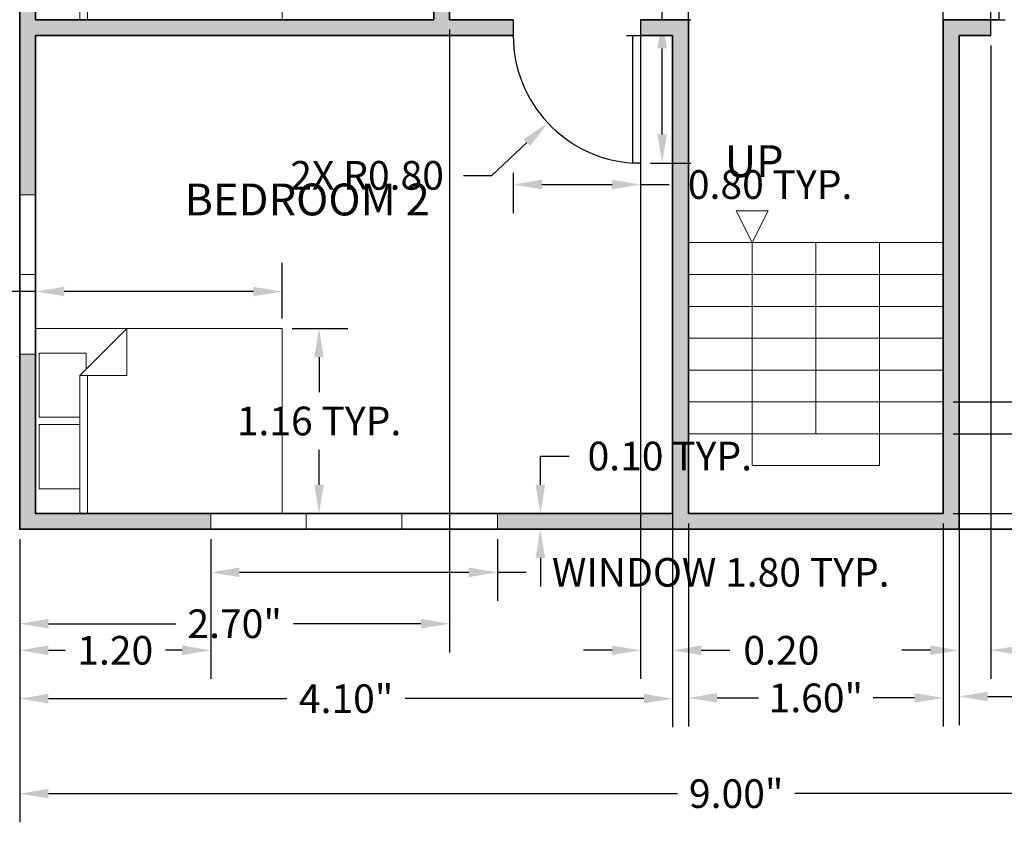
# Model space of a CAD drawing. Units: metres. Extents: x -1.9 to 13.1, y 0.9 to 14.8.
# Tile 2 of 7: x 1.2 to 7.4, y 0.9 to 5.9. Entities that reach past the tile are written whole.
import ezdxf

# ---------------------------------------------------------------- set-up
doc = ezdxf.new("R2010")
doc.units = ezdxf.units.M
doc.header["$MEASUREMENT"] = 0
for name, color, linetype, lineweight in [('A-ANNO-DIMS', 2, 'Continuous', 13), ('A-ANNO-SYMB', 7, 'Continuous', 18), ('A-ANNO-TEXT', 7, 'Continuous', 18), ('A-AREA-IDEN', 7, 'Continuous', 25), ('A-DOOR', 3, 'Continuous', 25), ('A-FLOR-STRS', 7, 'Continuous', 18), ('A-FURN', 8, 'Continuous', 18), ('A-GLAZ', 4, 'Continuous', 18), ('A-WALL', 7, 'Continuous', 35), ('A-WALL-PATT', 252, 'Continuous', 13)]:
    doc.layers.add(name, color=color, linetype=linetype, lineweight=lineweight)
doc.styles.get("Standard").update_dxf_attribs({"font": 'arial.ttf'})
doc.dimstyles.get("Standard").update_dxf_attribs({"dimtxt": 0.18, "dimasz": 0.18, "dimexe": 0.18, "dimexo": 0.0625, "dimgap": 0.09, "dimtad": 0, "dimtih": 1, "dimtoh": 1, "dimzin": 0, "dimdsep": 46, "dimlunit": 3, "dimtxsty": 'Standard', "dimcen": 0.09, "dimadec": 0, "dimazin": 0, "dimtfac": 1, "dimtofl": 0, "dimtmove": 0, "dimatfit": 3, "dimfxl": 1, "dimtolj": 1, "dimtzin": 0, "dimarcsym": 0})

# ---------------------------------------------------------------- blocks, each defined once
blk = doc.blocks.new('Bed - Queen')
for p, q in [((0, -80.00003), (0, 0)), ((0, 0), (59.99999, 0)), ((59.99999, 0), (59.99999, -80.00003)), ((7.99999, -1.2), (28.79998, -1.2)), ((7.99999, -14.4), (7.99999, -1.2)), ((28.79998, -1.2), (28.79998, -14.4)), ((31.19999, -1.2), (51.99999, -1.2)), ((31.19999, -14.4), (31.19999, -1.2)), ((51.99999, -1.2), (51.99999, -16.4)), ((0, -14.4), (44.8, -14.4)), ((59.99999, -29.6), (44.8, -14.4)), ((44.8, -14.4), (44.8, -29.6)), ((44.8, -16.8), (0, -16.8)), ((51.99999, -16.4), (46.79936, -16.4)), ((44.8, -29.6), (59.99999, -29.6)), ((59.99999, -80.00003), (0, -80.00003))]:
    blk.add_line(p, q)
blk = doc.blocks.new('*D8')
at = {"layer": 'A-ANNO-DIMS', "color": 0, "lineweight": -2, "transparency": 16777216}
for p, q in [((3.9038, 5.8339), (3.9038, 1.9238)), ((1.2038, 2.6339), (1.2038, 1.9238)), ((1.3838, 2.1038), (2.1841, 2.1038)), ((3.7238, 2.1038), (2.9236, 2.1038))]:
    blk.add_line(p, q, dxfattribs=at)
at = {"layer": 'A-ANNO-DIMS', "color": 0, "transparency": 16777216}
for points in [[(1.3838, 2.1338), (1.3838, 2.0738), (1.2038, 2.1038)], [(3.7238, 2.1338), (3.7238, 2.0738), (3.9038, 2.1038)]]:
    blk.add_solid(points, dxfattribs=at)
at = {"layer": 'Defpoints', "color": 0, "transparency": 16777216}
for p in [(3.9038, 5.8964), (1.2038, 2.6964), (3.9038, 2.1038)]:
    blk.add_point(p, dxfattribs=at)
at = {"layer": 'A-ANNO-DIMS', "color": 0, "transparency": 16777216, "insert": (2.5538, 2.1038), "char_height": 0.18, "attachment_point": 5}
blk.add_mtext('\\A1;2.70"', dxfattribs=at)
blk = doc.blocks.new('*D9')
at = {"layer": 'A-ANNO-DIMS', "color": 0, "lineweight": -2, "transparency": 16777216}
for p, q in [((5.3038, 2.7339), (5.3038, 1.4532)), ((1.2038, 2.6339), (1.2038, 1.4532)), ((1.3838, 1.6332), (2.882, 1.6332)), ((5.1238, 1.6332), (3.6257, 1.6332))]:
    blk.add_line(p, q, dxfattribs=at)
at = {"layer": 'A-ANNO-DIMS', "color": 0, "transparency": 16777216}
for points in [[(1.3838, 1.6632), (1.3838, 1.6032), (1.2038, 1.6332)], [(5.1238, 1.6632), (5.1238, 1.6032), (5.3038, 1.6332)]]:
    blk.add_solid(points, dxfattribs=at)
at = {"layer": 'Defpoints', "color": 0, "transparency": 16777216}
for p in [(5.3038, 2.7964), (1.2038, 2.6964), (5.3038, 1.6332)]:
    blk.add_point(p, dxfattribs=at)
at = {"layer": 'A-ANNO-DIMS', "color": 0, "transparency": 16777216, "insert": (3.2538, 1.6332), "char_height": 0.18, "attachment_point": 5}
blk.add_mtext('\\A1;4.10"', dxfattribs=at)
blk = doc.blocks.new('*D10')
at = {"layer": 'A-ANNO-DIMS', "color": 0, "lineweight": -2, "transparency": 16777216}
for p, q in [((5.4038, 2.7339), (5.4038, 1.4582)), ((7.0038, 2.7339), (7.0038, 1.4582)), ((5.5838, 1.6382), (5.8441, 1.6382)), ((6.8238, 1.6382), (6.5636, 1.6382))]:
    blk.add_line(p, q, dxfattribs=at)
at = {"layer": 'A-ANNO-DIMS', "color": 0, "transparency": 16777216}
for points in [[(5.5838, 1.6682), (5.5838, 1.6082), (5.4038, 1.6382)], [(6.8238, 1.6682), (6.8238, 1.6082), (7.0038, 1.6382)]]:
    blk.add_solid(points, dxfattribs=at)
at = {"layer": 'Defpoints', "color": 0, "transparency": 16777216}
for p in [(5.4038, 2.7964), (7.0038, 2.7964), (7.0038, 1.6382)]:
    blk.add_point(p, dxfattribs=at)
at = {"layer": 'A-ANNO-DIMS', "color": 0, "transparency": 16777216, "insert": (6.2038, 1.6382), "char_height": 0.18, "attachment_point": 5}
blk.add_mtext('\\A1;1.60"', dxfattribs=at)
blk = doc.blocks.new('*D11')
at = {"layer": 'A-ANNO-DIMS', "color": 0, "lineweight": -2, "transparency": 16777216}
for p, q in [((7.1038, 2.6339), (7.1038, 1.467)), ((10.2038, 2.6339), (10.2038, 1.467)), ((7.2838, 1.647), (8.2857, 1.647)), ((10.0238, 1.647), (9.022, 1.647))]:
    blk.add_line(p, q, dxfattribs=at)
at = {"layer": 'A-ANNO-DIMS', "color": 0, "transparency": 16777216}
for points in [[(7.2838, 1.677), (7.2838, 1.617), (7.1038, 1.647)], [(10.0238, 1.677), (10.0238, 1.617), (10.2038, 1.647)]]:
    blk.add_solid(points, dxfattribs=at)
at = {"layer": 'Defpoints', "color": 0, "transparency": 16777216}
for p in [(7.1038, 2.6964), (10.2038, 2.6964), (10.2038, 1.647)]:
    blk.add_point(p, dxfattribs=at)
at = {"layer": 'A-ANNO-DIMS', "color": 0, "transparency": 16777216, "insert": (8.6538, 1.647), "char_height": 0.18, "attachment_point": 5}
blk.add_mtext('\\A1;3.10"', dxfattribs=at)
blk = doc.blocks.new('*D12')
at = {"layer": 'A-ANNO-DIMS', "color": 0, "lineweight": -2, "transparency": 16777216}
for p, q in [((1.2038, 2.6339), (1.2038, 0.8568)), ((10.2038, 2.6339), (10.2038, 0.8568)), ((1.3838, 1.0368), (5.3356, 1.0368)), ((10.0238, 1.0368), (6.0721, 1.0368))]:
    blk.add_line(p, q, dxfattribs=at)
at = {"layer": 'A-ANNO-DIMS', "color": 0, "transparency": 16777216}
for points in [[(1.3838, 1.0668), (1.3838, 1.0068), (1.2038, 1.0368)], [(10.0238, 1.0668), (10.0238, 1.0068), (10.2038, 1.0368)]]:
    blk.add_solid(points, dxfattribs=at)
at = {"layer": 'Defpoints', "color": 0, "transparency": 16777216}
for p in [(1.2038, 2.6964), (10.2038, 2.6964), (10.2038, 1.0368)]:
    blk.add_point(p, dxfattribs=at)
at = {"layer": 'A-ANNO-DIMS', "color": 0, "transparency": 16777216, "insert": (5.7038, 1.0368), "char_height": 0.18, "attachment_point": 5}
blk.add_mtext('\\A1;9.00"', dxfattribs=at)
blk = doc.blocks.new('*D13')
at = {"layer": 'A-ANNO-DIMS', "color": 0, "lineweight": -2, "transparency": 16777216}
for p, q in [((7.1663, 13.6964), (12.9272, 13.6964)), ((12.7472, 13.5164), (12.7472, 8.3783)), ((12.7472, 2.8764), (12.7472, 8.0145)), ((10.2663, 2.6964), (12.9272, 2.6964))]:
    blk.add_line(p, q, dxfattribs=at)
at = {"layer": 'A-ANNO-DIMS', "color": 0, "transparency": 16777216}
for points in [[(12.7172, 13.5164), (12.7772, 13.5164), (12.7472, 13.6964)], [(12.7172, 2.8764), (12.7772, 2.8764), (12.7472, 2.6964)]]:
    blk.add_solid(points, dxfattribs=at)
at = {"layer": 'Defpoints', "color": 0, "transparency": 16777216}
for p in [(7.1038, 13.6964), (12.7472, 13.6964), (10.2038, 2.6964)]:
    blk.add_point(p, dxfattribs=at)
at = {"layer": 'A-ANNO-DIMS', "color": 0, "transparency": 16777216, "insert": (12.7472, 8.1964), "char_height": 0.18, "attachment_point": 5}
blk.add_mtext('\\A1;11.00"', dxfattribs=at)
blk = doc.blocks.new('*D20')
at = {"layer": 'A-ANNO-DIMS', "color": 0, "lineweight": -2, "transparency": 16777216}
for p, q in [((1.1413, 10.5964), (-1.7723, 10.5964)), ((-1.5923, 10.4164), (-1.5923, 6.8283)), ((-1.5923, 2.8764), (-1.5923, 6.4645)), ((1.1413, 2.6964), (-1.7723, 2.6964))]:
    blk.add_line(p, q, dxfattribs=at)
at = {"layer": 'A-ANNO-DIMS', "color": 0, "transparency": 16777216}
for points in [[(-1.6223, 10.4164), (-1.5623, 10.4164), (-1.5923, 10.5964)], [(-1.6223, 2.8764), (-1.5623, 2.8764), (-1.5923, 2.6964)]]:
    blk.add_solid(points, dxfattribs=at)
at = {"layer": 'Defpoints', "color": 0, "transparency": 16777216}
for p in [(1.2038, 10.5964), (-1.5923, 2.6964), (1.2038, 2.6964)]:
    blk.add_point(p, dxfattribs=at)
at = {"layer": 'A-ANNO-DIMS', "color": 0, "transparency": 16777216, "insert": (-1.5923, 6.6464), "char_height": 0.18, "attachment_point": 5}
blk.add_mtext('\\A1;7.90"', dxfattribs=at)
blk = doc.blocks.new('*D22')
at = {"layer": 'A-ANNO-DIMS', "color": 0, "lineweight": -2, "transparency": 16777216}
for p, q in [((1.1413, 9.2964), (-0.3896, 9.2964)), ((-0.2096, 9.1164), (-0.2096, 7.7756)), ((-0.2096, 6.0709), (-0.2096, 7.4117)), ((1.1413, 5.8909), (-0.3896, 5.8909))]:
    blk.add_line(p, q, dxfattribs=at)
at = {"layer": 'A-ANNO-DIMS', "color": 0, "transparency": 16777216}
for points in [[(-0.2396, 9.1164), (-0.1796, 9.1164), (-0.2096, 9.2964)], [(-0.2396, 6.0709), (-0.1796, 6.0709), (-0.2096, 5.8909)]]:
    blk.add_solid(points, dxfattribs=at)
at = {"layer": 'Defpoints', "color": 0, "transparency": 16777216}
for p in [(1.2038, 9.2964), (-0.2096, 5.8909), (1.2038, 5.8909)]:
    blk.add_point(p, dxfattribs=at)
at = {"layer": 'A-ANNO-DIMS', "color": 0, "transparency": 16777216, "insert": (-0.2096, 7.5936), "char_height": 0.18, "attachment_point": 5}
blk.add_mtext('\\A1;3.41"', dxfattribs=at)
blk = doc.blocks.new('*D23')
at = {"layer": 'A-ANNO-DIMS', "color": 0, "lineweight": -2, "transparency": 16777216}
for p, q in [((1.1413, 5.7874), (-0.4098, 5.7874)), ((-0.2298, 5.6074), (-0.2298, 4.4239)), ((-0.2298, 2.8764), (-0.2298, 4.0599)), ((1.1413, 2.6964), (-0.4098, 2.6964))]:
    blk.add_line(p, q, dxfattribs=at)
at = {"layer": 'A-ANNO-DIMS', "color": 0, "transparency": 16777216}
for points in [[(-0.2598, 5.6074), (-0.1998, 5.6074), (-0.2298, 5.7874)], [(-0.2598, 2.8764), (-0.1998, 2.8764), (-0.2298, 2.6964)]]:
    blk.add_solid(points, dxfattribs=at)
at = {"layer": 'Defpoints', "color": 0, "transparency": 16777216}
for p in [(1.2038, 5.7874), (-0.2298, 2.6964), (1.2038, 2.6964)]:
    blk.add_point(p, dxfattribs=at)
at = {"layer": 'A-ANNO-DIMS', "color": 0, "transparency": 16777216, "insert": (-0.2298, 4.2419), "char_height": 0.18, "attachment_point": 5}
blk.add_mtext('\\A1;3.09"', dxfattribs=at)
blk = doc.blocks.new('DOOR-800')
for p, q in [((0, 0.9), (0, 0.8)), ((0.8, 0.9), (0.8, 0.8)), ((0.75, 0), (0.75, 0.8)), ((0.75, 0.8), (0.8, 0.8)), ((0.8, 0.8), (0.8, 0)), ((0.8, 0), (0.75, 0))]:
    blk.add_line(p, q)
blk.add_arc((0.8017, 0.8), 0.8017, 180, 266.30478)
blk = doc.blocks.new('WIN-1000')
for p, q in [((0.1, 1), (0, 1)), ((0.1, 0.5), (0, 0.5)), ((0.1, 0), (0, 0))]:
    blk.add_line(p, q)
blk = doc.blocks.new('WIN-1800')
for p, q in [((0, 0.1), (0, 0)), ((0.6, 0.1), (0.6, 0)), ((1.2, 0.1), (1.2, 0)), ((1.8, 0.1), (1.8, 0))]:
    blk.add_line(p, q)
blk = doc.blocks.new('*D30')
at = {"layer": 'A-ANNO-DIMS', "color": 0, "lineweight": -2, "transparency": 16777216}
for p, q in [((2.4038, 2.6339), (2.4038, 2.2464)), ((4.2038, 2.6339), (4.2038, 2.2464)), ((2.5838, 2.4264), (4.0238, 2.4264)), ((4.2038, 2.4264), (4.3838, 2.4264))]:
    blk.add_line(p, q, dxfattribs=at)
at = {"layer": 'A-ANNO-DIMS', "color": 0, "transparency": 16777216}
for points in [[(2.5838, 2.4564), (2.5838, 2.3964), (2.4038, 2.4264)], [(4.0238, 2.4564), (4.0238, 2.3964), (4.2038, 2.4264)]]:
    blk.add_solid(points, dxfattribs=at)
at = {"layer": 'Defpoints', "color": 0, "transparency": 16777216}
for p in [(2.4038, 2.6964), (4.2038, 2.6964), (4.2038, 2.4264)]:
    blk.add_point(p, dxfattribs=at)
at = {"layer": 'A-ANNO-DIMS', "color": 0, "transparency": 16777216, "insert": (5.6071, 2.4264), "char_height": 0.18, "attachment_point": 5}
blk.add_mtext('\\A1;WINDOW 1.80 TYP.', dxfattribs=at)
blk = doc.blocks.new('*D31')
at = {"layer": 'A-ANNO-DIMS', "color": 0, "lineweight": -2, "transparency": 16777216}
for p, q in [((4.4738, 2.9764), (4.4738, 3.1564)), ((4.4738, 3.1564), (4.6538, 3.1564)), ((4.2663, 2.7964), (4.6538, 2.7964)), ((4.2663, 2.6964), (4.6538, 2.6964)), ((4.4738, 2.5164), (4.4738, 2.3364))]:
    blk.add_line(p, q, dxfattribs=at)
at = {"layer": 'A-ANNO-DIMS', "color": 0, "transparency": 16777216}
for points in [[(4.4438, 2.9764), (4.5038, 2.9764), (4.4738, 2.7964)], [(4.4438, 2.5164), (4.5038, 2.5164), (4.4738, 2.6964)]]:
    blk.add_solid(points, dxfattribs=at)
at = {"layer": 'Defpoints', "color": 0, "transparency": 16777216}
for p in [(4.2038, 2.7964), (4.4738, 2.7964), (4.2038, 2.6964)]:
    blk.add_point(p, dxfattribs=at)
at = {"layer": 'A-ANNO-DIMS', "color": 0, "transparency": 16777216, "insert": (5.2868, 3.1564), "char_height": 0.18, "attachment_point": 5}
blk.add_mtext('\\A1;0.10 TYP.', dxfattribs=at)
blk = doc.blocks.new('*D34')
at = {"layer": 'A-ANNO-DIMS', "color": 0, "lineweight": -2, "transparency": 16777216}
for p, q in [((5.2388, 5.8964), (5.2388, 6.0764)), ((5.2388, 6.0764), (5.4188, 6.0764)), ((5.1663, 5.8964), (5.4188, 5.8964)), ((5.2388, 5.1764), (5.2388, 5.7164)), ((5.1663, 4.9964), (5.4188, 4.9964))]:
    blk.add_line(p, q, dxfattribs=at)
at = {"layer": 'A-ANNO-DIMS', "color": 0, "transparency": 16777216}
for points in [[(5.2088, 5.7164), (5.2688, 5.7164), (5.2388, 5.8964)], [(5.2088, 5.1764), (5.2688, 5.1764), (5.2388, 4.9964)]]:
    blk.add_solid(points, dxfattribs=at)
at = {"layer": 'Defpoints', "color": 0, "transparency": 16777216}
for p in [(5.1038, 5.8964), (5.2388, 5.8964), (5.1038, 4.9964)]:
    blk.add_point(p, dxfattribs=at)
at = {"layer": 'A-ANNO-DIMS', "color": 0, "transparency": 16777216, "insert": (6.4594, 6.0764), "char_height": 0.18, "attachment_point": 5}
blk.add_mtext('\\A1;DOOR 0.90 TYP.', dxfattribs=at)
blk = doc.blocks.new('*D35')
at = {"layer": 'A-ANNO-DIMS', "color": 0, "lineweight": -2, "transparency": 16777216}
for p, q in [((4.3038, 4.9339), (4.3038, 4.6814)), ((5.1038, 4.9339), (5.1038, 4.6814)), ((4.4838, 4.8614), (4.9238, 4.8614)), ((5.1038, 4.8614), (5.2838, 4.8614))]:
    blk.add_line(p, q, dxfattribs=at)
at = {"layer": 'A-ANNO-DIMS', "color": 0, "transparency": 16777216}
for points in [[(4.4838, 4.8914), (4.4838, 4.8314), (4.3038, 4.8614)], [(4.9238, 4.8914), (4.9238, 4.8314), (5.1038, 4.8614)]]:
    blk.add_solid(points, dxfattribs=at)
at = {"layer": 'Defpoints', "color": 0, "transparency": 16777216}
for p in [(4.3038, 4.9964), (5.1038, 4.9964), (5.1038, 4.8614)]:
    blk.add_point(p, dxfattribs=at)
at = {"layer": 'A-ANNO-DIMS', "color": 0, "transparency": 16777216, "insert": (5.9168, 4.8614), "char_height": 0.18, "attachment_point": 5}
blk.add_mtext('\\A1;0.80 TYP.', dxfattribs=at)
blk = doc.blocks.new('*D36')
at = {"layer": 'A-ANNO-DIMS', "color": 0, "lineweight": -2, "transparency": 16777216}
for p, q in [((1.3038, 4.0198), (1.3038, 4.3694)), ((2.8517, 4.0198), (2.8517, 4.3694)), ((1.3038, 4.1894), (1.1238, 4.1894)), ((2.6717, 4.1894), (1.4838, 4.1894))]:
    blk.add_line(p, q, dxfattribs=at)
at = {"layer": 'A-ANNO-DIMS', "color": 0, "transparency": 16777216}
for points in [[(1.4838, 4.2194), (1.4838, 4.1594), (1.3038, 4.1894)], [(2.6717, 4.2194), (2.6717, 4.1594), (2.8517, 4.1894)]]:
    blk.add_solid(points, dxfattribs=at)
at = {"layer": 'Defpoints', "color": 0, "transparency": 16777216}
for p in [(1.3038, 4.1894), (1.3038, 3.9573), (2.8517, 3.9573)]:
    blk.add_point(p, dxfattribs=at)
at = {"layer": 'A-ANNO-DIMS', "color": 0, "transparency": 16777216, "insert": (0.2014, 4.1894), "char_height": 0.18, "attachment_point": 5}
blk.add_mtext('\\A1;BED 1.55 TYP.', dxfattribs=at)
blk = doc.blocks.new('*D37')
at = {"layer": 'A-ANNO-DIMS', "color": 0, "lineweight": -2, "transparency": 16777216}
for p, q in [((2.9142, 3.9573), (3.2639, 3.9573)), ((3.0839, 3.7773), (3.0839, 3.5587)), ((3.0839, 2.9764), (3.0839, 3.1949)), ((2.9142, 2.7964), (3.2639, 2.7964))]:
    blk.add_line(p, q, dxfattribs=at)
at = {"layer": 'A-ANNO-DIMS', "color": 0, "transparency": 16777216}
for points in [[(3.0539, 3.7773), (3.1139, 3.7773), (3.0839, 3.9573)], [(3.0539, 2.9764), (3.1139, 2.9764), (3.0839, 2.7964)]]:
    blk.add_solid(points, dxfattribs=at)
at = {"layer": 'Defpoints', "color": 0, "transparency": 16777216}
for p in [(2.8517, 3.9573), (3.0839, 3.9573), (2.8517, 2.7964)]:
    blk.add_point(p, dxfattribs=at)
at = {"layer": 'A-ANNO-DIMS', "color": 0, "transparency": 16777216, "insert": (3.0839, 3.3768), "char_height": 0.18, "attachment_point": 5}
blk.add_mtext('\\A1;1.16 TYP.', dxfattribs=at)
blk = doc.blocks.new('*D50')
at = {"layer": 'A-ANNO-DIMS', "color": 0, "lineweight": -2, "transparency": 16777216}
for p, q in [((1.203847, 2.633878), (1.203847, 1.756878)), ((2.403847, 2.633878), (2.403847, 1.756878)), ((1.383847, 1.936878), (1.488847, 1.936878)), ((2.223847, 1.936878), (2.118847, 1.936878))]:
    blk.add_line(p, q, dxfattribs=at)
at = {"layer": 'A-ANNO-DIMS', "color": 0, "transparency": 16777216}
for points in [[(1.383847, 1.966878), (1.383847, 1.906878), (1.203847, 1.936878)], [(2.223847, 1.966878), (2.223847, 1.906878), (2.403847, 1.936878)]]:
    blk.add_solid(points, dxfattribs=at)
at = {"layer": 'Defpoints', "color": 0, "transparency": 16777216}
for p in [(1.203847, 2.696378), (2.403847, 2.696378), (2.403847, 1.936878)]:
    blk.add_point(p, dxfattribs=at)
at = {"layer": 'A-ANNO-DIMS', "color": 0, "transparency": 16777216, "insert": (1.803847, 1.936878), "char_height": 0.18, "attachment_point": 5}
blk.add_mtext('\\A1;1.20', dxfattribs=at)
blk = doc.blocks.new('*D59')
at = {"layer": 'A-ANNO-DIMS', "color": 0, "lineweight": -2, "transparency": 16777216}
for p, q in [((7.1038, 5.7339), (7.1038, 1.7569)), ((7.3038, 5.7339), (7.3038, 1.7569)), ((6.9238, 1.9369), (6.7438, 1.9369)), ((7.4838, 1.9369), (7.6638, 1.9369))]:
    blk.add_line(p, q, dxfattribs=at)
at = {"layer": 'A-ANNO-DIMS', "color": 0, "transparency": 16777216}
for points in [[(6.9238, 1.9669), (6.9238, 1.9069), (7.1038, 1.9369)], [(7.4838, 1.9669), (7.4838, 1.9069), (7.3038, 1.9369)]]:
    blk.add_solid(points, dxfattribs=at)
at = {"layer": 'Defpoints', "color": 0, "transparency": 16777216}
for p in [(7.1038, 5.7964), (7.3038, 5.7964), (7.3038, 1.9369)]:
    blk.add_point(p, dxfattribs=at)
at = {"layer": 'A-ANNO-DIMS', "color": 0, "transparency": 16777216, "insert": (7.9873, 1.9369), "char_height": 0.18, "attachment_point": 5}
blk.add_mtext('\\A1;0.20', dxfattribs=at)
blk = doc.blocks.new('*D64')
at = {"layer": 'A-ANNO-DIMS', "color": 0, "lineweight": -2, "transparency": 16777216}
for p, q in [((5.1038, 5.7339), (5.1038, 1.7569)), ((5.3038, 5.7339), (5.3038, 1.7569)), ((4.9238, 1.9369), (4.7438, 1.9369)), ((5.4838, 1.9369), (5.6638, 1.9369))]:
    blk.add_line(p, q, dxfattribs=at)
at = {"layer": 'A-ANNO-DIMS', "color": 0, "transparency": 16777216}
for points in [[(4.9238, 1.9669), (4.9238, 1.9069), (5.1038, 1.9369)], [(5.4838, 1.9669), (5.4838, 1.9069), (5.3038, 1.9369)]]:
    blk.add_solid(points, dxfattribs=at)
at = {"layer": 'Defpoints', "color": 0, "transparency": 16777216}
for p in [(5.1038, 5.7964), (5.3038, 5.7964), (5.3038, 1.9369)]:
    blk.add_point(p, dxfattribs=at)
at = {"layer": 'A-ANNO-DIMS', "color": 0, "transparency": 16777216, "insert": (5.9873, 1.9369), "char_height": 0.18, "attachment_point": 5}
blk.add_mtext('\\A1;0.20', dxfattribs=at)
blk = doc.blocks.new('*D66')
at = {"layer": 'A-ANNO-DIMS', "color": 0, "lineweight": -2, "transparency": 16777216}
for p, q in [((5.403847, 4.558878), (5.403847, 14.635878)), ((7.003847, 4.558878), (7.003847, 14.635878)), ((5.583847, 14.455878), (5.888847, 14.455878)), ((6.823847, 14.455878), (6.518847, 14.455878))]:
    blk.add_line(p, q, dxfattribs=at)
at = {"layer": 'A-ANNO-DIMS', "color": 0, "transparency": 16777216}
for points in [[(5.583847, 14.485878), (5.583847, 14.425878), (5.403847, 14.455878)], [(6.823847, 14.485878), (6.823847, 14.425878), (7.003847, 14.455878)]]:
    blk.add_solid(points, dxfattribs=at)
at = {"layer": 'Defpoints', "color": 0, "transparency": 16777216}
for p in [(7.003847, 14.455878), (5.403847, 4.496378), (7.003847, 4.496378)]:
    blk.add_point(p, dxfattribs=at)
at = {"layer": 'A-ANNO-DIMS', "color": 0, "transparency": 16777216, "insert": (6.203847, 14.455878), "char_height": 0.18, "attachment_point": 5}
blk.add_mtext('\\A1;1.60', dxfattribs=at)
blk = doc.blocks.new('*D67')
at = {"layer": 'A-ANNO-DIMS', "color": 0, "lineweight": -2, "transparency": 16777216}
for p, q in [((10.9633, 3.6764), (10.9633, 3.8564)), ((7.0663, 3.4964), (11.1433, 3.4964)), ((7.0663, 3.2964), (11.1433, 3.2964)), ((10.9633, 3.1164), (10.9633, 2.9364)), ((10.9633, 2.9364), (10.7833, 2.9364))]:
    blk.add_line(p, q, dxfattribs=at)
at = {"layer": 'A-ANNO-DIMS', "color": 0, "transparency": 16777216}
for points in [[(10.9333, 3.6764), (10.9933, 3.6764), (10.9633, 3.4964)], [(10.9333, 3.1164), (10.9933, 3.1164), (10.9633, 3.2964)]]:
    blk.add_solid(points, dxfattribs=at)
at = {"layer": 'Defpoints', "color": 0, "transparency": 16777216}
for p in [(7.0038, 3.4964), (7.0038, 3.2964), (10.9633, 3.2964)]:
    blk.add_point(p, dxfattribs=at)
at = {"layer": 'A-ANNO-DIMS', "color": 0, "transparency": 16777216, "insert": (10.4599, 2.9364), "char_height": 0.18, "attachment_point": 5}
blk.add_mtext('\\A1;0.20', dxfattribs=at)
blk = doc.blocks.new('*D68')
at = {"layer": 'A-ANNO-DIMS', "color": 0, "lineweight": -2, "transparency": 16777216}
for p, q in [((10.963347, 3.476378), (10.963347, 3.656378)), ((7.066347, 3.296378), (11.143347, 3.296378)), ((7.066347, 2.796378), (11.143347, 2.796378)), ((10.963347, 2.616378), (10.963347, 2.436378))]:
    blk.add_line(p, q, dxfattribs=at)
at = {"layer": 'A-ANNO-DIMS', "color": 0, "transparency": 16777216}
for points in [[(10.933347, 3.476378), (10.993347, 3.476378), (10.963347, 3.296378)], [(10.933347, 2.616378), (10.993347, 2.616378), (10.963347, 2.796378)]]:
    blk.add_solid(points, dxfattribs=at)
at = {"layer": 'Defpoints', "color": 0, "transparency": 16777216}
for p in [(7.003847, 3.296378), (7.003847, 2.796378), (10.963347, 2.796378)]:
    blk.add_point(p, dxfattribs=at)
at = {"layer": 'A-ANNO-DIMS', "color": 0, "transparency": 16777216, "insert": (10.963347, 3.046378), "char_height": 0.18, "attachment_point": 5}
blk.add_mtext('\\A1;0.50', dxfattribs=at)
blk = doc.blocks.new('*D75')
at = {"layer": 'A-ANNO-DIMS', "color": 0, "lineweight": -2, "transparency": 16777216}
for p, q in [((8.4637, 7.0002), (8.1587, 6.7103)), ((8.6437, 7.0002), (8.4637, 7.0002)), ((7.3025, 5.8064), (7.3025, 5.9864)), ((7.2125, 5.8964), (7.3925, 5.8964))]:
    blk.add_line(p, q, dxfattribs=at)
at = {"layer": 'A-ANNO-DIMS', "color": 0, "transparency": 16777216}
blk.add_solid([(8.1381, 6.732), (8.1794, 6.6885), (8.0283, 6.5863)], dxfattribs=at)
at = {"layer": 'Defpoints', "color": 0, "transparency": 16777216}
for p in [(8.0283, 6.5863), (7.3025, 5.8964)]:
    blk.add_point(p, dxfattribs=at)
at = {"layer": 'A-ANNO-DIMS', "color": 0, "transparency": 16777216, "insert": (9.0533, 7.0002), "char_height": 0.18, "attachment_point": 5}
blk.add_mtext('\\A1;R1.00', dxfattribs=at)
blk = doc.blocks.new('*D76')
at = {"layer": 'A-ANNO-DIMS', "color": 0, "lineweight": -2, "transparency": 16777216}
for p, q in [((5.1055, 5.7064), (5.1055, 5.8864)), ((5.0155, 5.7964), (5.1955, 5.7964)), ((4.1701, 4.9188), (4.3896, 5.1247)), ((3.9901, 4.9188), (4.1701, 4.9188))]:
    blk.add_line(p, q, dxfattribs=at)
at = {"layer": 'A-ANNO-DIMS', "color": 0, "transparency": 16777216}
blk.add_solid([(4.3691, 5.1466), (4.4101, 5.1028), (4.5209, 5.2479)], dxfattribs=at)
at = {"layer": 'Defpoints', "color": 0, "transparency": 16777216}
for p in [(5.1055, 5.7964), (4.5209, 5.2479)]:
    blk.add_point(p, dxfattribs=at)
at = {"layer": 'A-ANNO-DIMS', "color": 0, "transparency": 16777216, "insert": (3.3856, 4.9188), "char_height": 0.18, "attachment_point": 5}
blk.add_mtext('\\A1;2X R0.80', dxfattribs=at)

msp = doc.modelspace()

# ---------------------------------------------------------------- linework, layer by layer
at = {"layer": 'A-ANNO-SYMB'}
msp.add_lwpolyline([(5.9038, 4.6964), (5.8038, 4.6964), (5.7038, 4.6964), (5.8038, 4.4964)], close=True, dxfattribs=at)
at = {"layer": 'A-DOOR'}
for p, q in [((7.3038, 5.8964), (7.3038, 6.8964)), ((7.3538, 6.8964), (7.3538, 5.8964)), ((7.3038, 5.7964), (7.3038, 5.8964)), ((7.3538, 5.8964), (7.3038, 5.8964))]:
    msp.add_line(p, q, dxfattribs=at)
msp.add_arc((7.3025, 5.8964), 1.0013, 0, 87.0624, dxfattribs=at)
at = {"layer": 'A-FLOR-STRS'}
for p, q in [((5.4038, 4.4964), (7.0038, 4.4964)), ((5.8038, 4.4964), (5.8038, 3.0964)), ((6.2038, 4.4964), (6.2038, 3.2964)), ((6.6038, 4.4964), (6.6038, 3.0964)), ((5.4038, 4.2964), (7.0038, 4.2964)), ((5.4038, 4.0964), (7.0038, 4.0964)), ((5.4038, 3.8964), (7.0038, 3.8964)), ((5.4038, 3.6964), (7.0038, 3.6964)), ((5.4038, 3.4964), (7.0038, 3.4964)), ((5.4038, 3.2964), (7.0038, 3.2964)), ((5.8038, 3.0964), (6.6038, 3.0964))]:
    msp.add_line(p, q, dxfattribs=at)
at = {"layer": 'A-WALL'}
for p, q in [((1.3038, 9.2964), (1.3038, 5.8964)), ((3.8038, 8.2964), (3.8038, 5.8964)), ((3.9038, 8.2964), (3.9038, 5.8964)), ((1.3038, 5.8964), (3.8038, 5.8964)), ((3.9038, 5.8964), (4.3038, 5.8964)), ((5.1038, 5.8964), (5.4038, 5.8964)), ((5.4038, 5.8964), (5.4038, 2.7964)), ((7.0038, 2.7964), (7.0038, 5.8964)), ((7.0038, 5.8964), (7.3038, 5.8964)), ((1.3038, 5.7964), (4.3038, 5.7964)), ((1.3038, 5.7964), (1.3038, 2.7964)), ((5.1038, 5.7964), (5.3038, 5.7964)), ((5.3038, 5.7964), (5.3038, 2.7964)), ((7.1038, 2.6964), (7.1038, 5.7964)), ((7.1038, 5.7964), (7.3038, 5.7964)), ((1.3038, 2.7964), (5.3038, 2.7964)), ((5.4038, 2.7964), (7.0038, 2.7964))]:
    msp.add_line(p, q, dxfattribs=at)
msp.add_lwpolyline([(1.2038, 10.5964), (1.2038, 2.6964), (10.2038, 2.6964), (10.2038, 10.5964)], dxfattribs=at)
at = {"layer": 'A-WALL-PATT'}
for points in [[(3.8038, 5.8964), (3.9038, 5.8964), (3.8038, 8.2964), (3.9038, 8.2964)], [(1.2038, 4.7964), (1.3038, 4.7964), (1.2038, 6.7785), (1.3038, 6.7785)], [(1.3038, 5.8964), (1.3038, 5.7964), (4.3038, 5.8964), (4.3038, 5.7964)], [(5.3038, 5.7964), (5.4038, 5.8964), (5.1038, 5.7964), (5.1038, 5.8964)], [(5.3038, 2.7964), (5.4038, 2.6964), (5.3038, 5.7964), (5.4038, 5.8964)], [(7.3038, 5.8964), (7.3038, 5.7964), (7.0038, 5.8964), (7.1038, 5.7964)], [(7.0038, 5.8964), (7.1038, 5.7964), (7.0038, 2.7964), (7.1038, 2.6964)], [(1.2038, 2.6964), (1.3038, 2.7964), (1.2038, 3.7964), (1.3038, 3.7964)], [(2.4038, 2.6964), (2.4038, 2.7964), (1.2038, 2.6964), (1.3038, 2.7964)], [(4.2038, 2.7964), (4.2038, 2.6964), (5.3038, 2.7964), (5.4038, 2.6964)], [(7.0038, 2.7964), (7.1038, 2.6964), (5.4038, 2.7964), (5.4038, 2.6964)]]:
    msp.add_solid(points, dxfattribs=at)

# ---------------------------------------------------------------- block references
at = {"layer": 'A-DOOR'}
msp.add_blockref('DOOR-800', (4.3038, 4.9964), dxfattribs=at)
at = {"layer": 'A-FURN', "xscale": 0.0193482099346659, "yscale": 0.0193482099346659, "zscale": 0.0193482099346659, "rotation": 90}
for p in [(1.3038, 5.8964), (1.3038, 2.7964)]:
    msp.add_blockref('Bed - Queen', p, dxfattribs=at)
at = {"layer": 'A-GLAZ'}
for name, p in [('WIN-1000', (1.2038, 3.7964)), ('WIN-1800', (2.4038, 2.6964))]:
    msp.add_blockref(name, p, dxfattribs=at)

# ---------------------------------------------------------------- texts
at = {"layer": 'A-ANNO-TEXT', "insert": (5.6141, 5.1084), "char_height": 0.2, "attachment_point": 1}
msp.add_mtext_dynamic_manual_height_columns('\\pxqc;UP', width=0.405496, gutter_width=1, heights=[0], dxfattribs=at)
at = {"layer": 'A-AREA-IDEN', "insert": (2.1612, 4.8674), "char_height": 0.2, "attachment_point": 1}
msp.add_mtext_dynamic_manual_height_columns('\\pxqc;BEDROOM 2', width=1.695526, gutter_width=1, heights=[0], dxfattribs=at)

# ---------------------------------------------------------------- dimensions: what is measured, and where the dimension line sits
at = {"layer": 'A-ANNO-DIMS'}
for base, p1, p2, override, picture, middle in [((7.0038, 14.4559), (5.4038, 4.4964), (7.0038, 4.4964), {"dimdec": 2, "dimlfac": 1, "dimrnd": 0, "dimzin": 0, "dimdsep": 46, "dimlunit": 2}, '*D66', (6.2038, 14.4559)), ((3.9038, 2.1038), (1.2038, 2.6964), (3.9038, 5.8964), {"dimclrd": 0, "dimclre": 0, "dimclrt": 0}, '*D8', (2.5538, 2.1038)), ((5.3038, 1.9369), (5.1038, 5.7964), (5.3038, 5.7964), {"dimdec": 2, "dimlfac": 1, "dimrnd": 0, "dimzin": 0, "dimdsep": 46, "dimlunit": 2}, '*D64', (5.9873, 1.9369)), ((7.3038, 1.9369), (7.1038, 5.7964), (7.3038, 5.7964), {"dimdec": 2, "dimlfac": 1, "dimrnd": 0, "dimzin": 0, "dimdsep": 46, "dimlunit": 2}, '*D59', (7.9873, 1.9369)), ((5.3038, 1.6332), (1.2038, 2.6964), (5.3038, 2.7964), {"dimclrd": 0, "dimclre": 0, "dimclrt": 0}, '*D9', (3.2538, 1.6332)), ((7.0038, 1.6382), (5.4038, 2.7964), (7.0038, 2.7964), {"dimclrd": 0, "dimclre": 0, "dimclrt": 0}, '*D10', (6.2038, 1.6382)), ((10.2038, 1.0368), (1.2038, 2.6964), (10.2038, 2.6964), {"dimclrd": 0, "dimclre": 0, "dimclrt": 0}, '*D12', (5.7038, 1.0368)), ((2.4038, 1.9369), (1.2038, 2.6964), (2.4038, 2.6964), {"dimdec": 2, "dimlfac": 1, "dimrnd": 0, "dimzin": 0, "dimdsep": 46, "dimlunit": 2}, '*D50', (1.8038, 1.9369)), ((10.2038, 1.647), (7.1038, 2.6964), (10.2038, 2.6964), {"dimclrd": 0, "dimclre": 0, "dimclrt": 0}, '*D11', (8.6538, 1.647))]:
    dim = msp.add_linear_dim(base=base, p1=p1, p2=p2, dimstyle='Standard', override=override, dxfattribs=at)
    dim.commit()
    dim.dimension.update_dxf_attribs({"geometry": picture, "text_midpoint": middle})
for base, p1, p2, override, picture, middle in [((12.7472, 13.6964), (10.2038, 2.6964), (7.1038, 13.6964), {"dimclrd": 0, "dimclre": 0, "dimclrt": 0}, '*D13', (12.7472, 8.1964)), ((-1.5923, 2.6964), (1.2038, 10.5964), (1.2038, 2.6964), {"dimclrd": 0, "dimclre": 0, "dimclrt": 0}, '*D20', (-1.5923, 6.6464)), ((-0.2096, 5.8909), (1.2038, 9.2964), (1.2038, 5.8909), {"dimclrd": 0, "dimclre": 0, "dimclrt": 0}, '*D22', (-0.2096, 7.5936)), ((-0.2298, 2.6964), (1.2038, 5.7874), (1.2038, 2.6964), {"dimclrd": 0, "dimclre": 0, "dimclrt": 0}, '*D23', (-0.2298, 4.2419)), ((10.9633, 3.2964), (7.0038, 3.4964), (7.0038, 3.2964), {"dimdec": 2, "dimlfac": 1, "dimrnd": 0, "dimzin": 0, "dimdsep": 46, "dimlunit": 2}, '*D67', (10.4599, 2.9364)), ((10.9633, 2.7964), (7.0038, 3.2964), (7.0038, 2.7964), {"dimdec": 2, "dimlfac": 1, "dimrnd": 0, "dimzin": 0, "dimdsep": 46, "dimlunit": 2}, '*D68', (10.9633, 3.0464))]:
    dim = msp.add_linear_dim(base=base, p1=p1, p2=p2, angle=90, dimstyle='Standard', override=override, dxfattribs=at)
    dim.commit()
    dim.dimension.update_dxf_attribs({"geometry": picture, "text_midpoint": middle})
dim = msp.add_radius_dim(center=(7.3025, 5.8964), mpoint=(8.0283, 6.5863), dimstyle='Standard', override={"dimdec": 2, "dimlfac": 1, "dimrnd": 0, "dimzin": 0, "dimdsep": 46, "dimlunit": 2}, dxfattribs=at)
dim.commit()
dim.dimension.update_dxf_attribs({"geometry": '*D75', "text_midpoint": (9.0533, 7.0002), "dimtype": 164})
for base, p1, p2, angle, text, picture, middle in [((5.2388, 5.8964), (5.1038, 4.9964), (5.1038, 5.8964), 90, 'DOOR <> TYP.', '*D34', (6.4594, 6.0764)), ((1.3038, 4.1894), (2.8517, 3.9573), (1.3038, 3.9573), 180, 'BED <> TYP.', '*D36', (0.2014, 4.1894)), ((3.0839, 3.9573), (2.8517, 2.7964), (2.8517, 3.9573), 90, '<> TYP.', '*D37', (3.0839, 3.3768)), ((4.4738, 2.7964), (4.2038, 2.6964), (4.2038, 2.7964), 90, '<> TYP.', '*D31', (5.2868, 3.1564))]:
    dim = msp.add_linear_dim(base=base, p1=p1, p2=p2, angle=angle, text=text, dimstyle='Standard', override={"dimdec": 2, "dimlfac": 1, "dimrnd": 0, "dimzin": 0, "dimdsep": 46, "dimlunit": 2}, dxfattribs=at)
    dim.commit()
    dim.dimension.update_dxf_attribs({"geometry": picture, "text_midpoint": middle})
dim = msp.add_radius_dim(center=(5.1055, 5.7964), mpoint=(4.5209, 5.2479), text='2X <>', dimstyle='Standard', override={"dimdec": 2, "dimlfac": 1, "dimrnd": 0, "dimzin": 0, "dimdsep": 46, "dimlunit": 2}, dxfattribs=at)
dim.commit()
dim.dimension.update_dxf_attribs({"geometry": '*D76', "text_midpoint": (3.3856, 4.9188), "dimtype": 164})
for base, p1, p2, text, picture, middle in [((5.1038, 4.8614), (4.3038, 4.9964), (5.1038, 4.9964), '<> TYP.', '*D35', (5.9168, 4.8614)), ((4.2038, 2.4264), (2.4038, 2.6964), (4.2038, 2.6964), 'WINDOW <> TYP.', '*D30', (5.6071, 2.4264))]:
    dim = msp.add_linear_dim(base=base, p1=p1, p2=p2, text=text, dimstyle='Standard', override={"dimdec": 2, "dimlfac": 1, "dimrnd": 0, "dimzin": 0, "dimdsep": 46, "dimlunit": 2}, dxfattribs=at)
    dim.commit()
    dim.dimension.update_dxf_attribs({"geometry": picture, "text_midpoint": middle})

doc.saveas('drawing.dxf')
